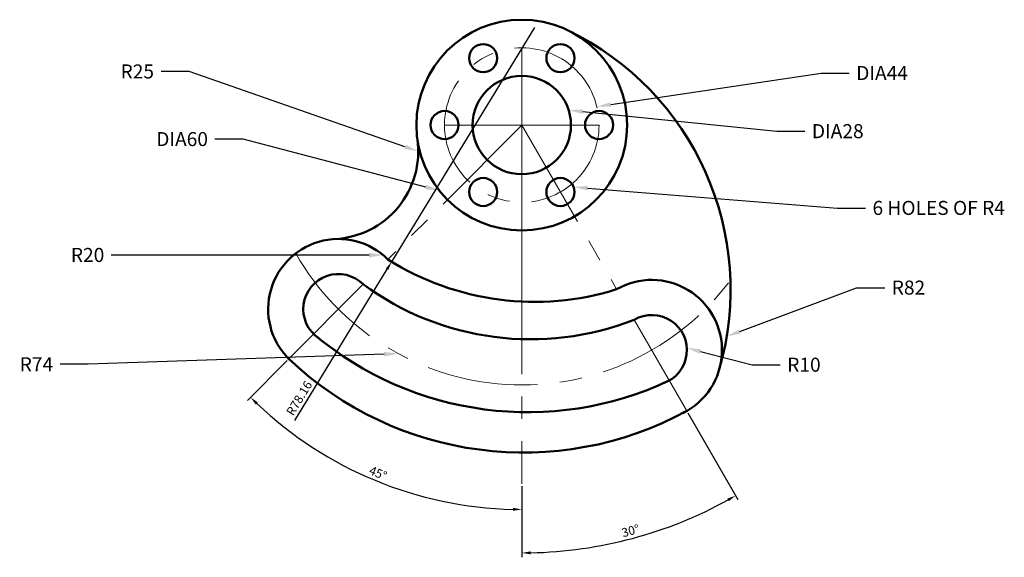
# Model space of a CAD drawing. Units: millimetres. Extents: x 3012 to 3292, y 2052 to 2205.
import ezdxf
from ezdxf import colors
from ezdxf.entities.mleader import LeaderData, LeaderLine
from ezdxf.math import Vec2, Vec3

# ---------------------------------------------------------------- set-up
doc = ezdxf.new("R2010")
doc.units = ezdxf.units.MM
doc.linetypes.add('CENTER', pattern=[50.8, 31.75, -6.35, 6.35, -6.35])
for name, color, linetype, lineweight in [('M-CNTR', 4, 'CENTER', 18), ('M-DIMS', 2, 'Continuous', 25), ('M-OUTL', 7, 'Continuous', 50)]:
    doc.layers.add(name, color=color, linetype=linetype, lineweight=lineweight)
doc.styles.get("Standard").update_dxf_attribs({"font": 'arial.ttf'})
doc.dimstyles.new('ISO-25', dxfattribs={"dimtxt": 2.5, "dimasz": 2.5, "dimexe": 1.25, "dimexo": 0.625, "dimtad": 1, "dimtxsty": 'Standard', "dimcen": 2.5, "dimadec": 0, "dimazin": 0, "dimtfac": 1, "dimtmove": 0, "dimatfit": 3, "dimfxl": 1, "dimarcsym": 0})

# ---------------------------------------------------------------- blocks, each defined once
blk = doc.blocks.new('*U1')
blk.add_circle((0, 0), 4)
blk = doc.blocks.new('*U2')
at = {"layer": 'M-OUTL', "color": 0, "linetype": 'ByBlock', "lineweight": -2, "transparency": 16777216}
for p, rotation in [((3143.61, 2193.94), 300), ((3165.61, 2193.94), 240), ((3176.61, 2174.89), 180), ((3143.61, 2155.83), 59.99999999999999), ((3165.61, 2155.83), 119.9999999999999)]:
    blk.add_blockref('*U1', p, dxfattribs=dict(at, rotation=rotation))
blk.add_blockref('*U1', (3132.61, 2174.89), dxfattribs=at)
blk = doc.blocks.new('*D3')
at = {"layer": 'Defpoints', "color": 0, "transparency": 16777216}
for p in [(3154.61, 2135.71), (3109.44, 2129.55), (3088.27, 2108.29), (3100.01, 2080.03), (3154.61, 2072.72)]:
    blk.add_point(p, dxfattribs=at)
at = {"layer": 'M-DIMS', "color": 0, "lineweight": -2, "transparency": 16777216}
for p, q in [((3087.83, 2107.85), (3076.49, 2096.46)), ((3154.61, 2072.1), (3154.61, 2064.19))]:
    blk.add_line(p, q, dxfattribs=at)
blk.add_arc((3154.61, 2174.89), 109.45, 226.4177, 268.6912, dxfattribs=at)
at = {"layer": 'M-DIMS', "color": 0, "transparency": 16777216}
for points in [[(3078.87, 2095.31), (3079.45, 2095.9), (3077.37, 2097.35)], [(3152.12, 2065.89), (3152.11, 2065.05), (3154.61, 2065.44)]]:
    blk.add_solid(points, dxfattribs=at)
at = {"layer": 'M-DIMS', "color": 0, "transparency": 16777216, "insert": (3113.55, 2075.49), "char_height": 2.5, "attachment_point": 5, "rotation": 337.5545}
blk.add_mtext('45°', dxfattribs=at)
blk = doc.blocks.new('*D4')
at = {"layer": 'Defpoints', "color": 0, "transparency": 16777216}
for p in [(3154.61, 2135.71), (3186.61, 2119.46), (3201.61, 2093.48), (3154.61, 2072.72), (3175.77, 2054.91)]:
    blk.add_point(p, dxfattribs=at)
at = {"layer": 'M-DIMS', "color": 0, "lineweight": -2, "transparency": 16777216}
for p, q in [((3201.93, 2092.94), (3216.15, 2068.3)), ((3154.61, 2072.1), (3154.61, 2051.81))]:
    blk.add_line(p, q, dxfattribs=at)
blk.add_arc((3154.61, 2174.89), 121.83, 271.1758, 298.8242, dxfattribs=at)
at = {"layer": 'M-DIMS', "color": 0, "transparency": 16777216}
for points in [[(3213.14, 2068.52), (3213.55, 2067.79), (3215.53, 2069.38)], [(3157.12, 2052.67), (3157.11, 2053.5), (3154.61, 2053.06)]]:
    blk.add_solid(points, dxfattribs=at)
at = {"layer": 'M-DIMS', "color": 0, "transparency": 16777216, "insert": (3185.65, 2059.05), "char_height": 2.5, "attachment_point": 5, "rotation": 15}
blk.add_mtext('30°', dxfattribs=at)
blk = doc.blocks.new('*D5')
at = {"layer": 'Defpoints', "color": 0, "transparency": 16777216}
for p in [(3158.25, 2202.71), (3117.55, 2135.98)]:
    blk.add_point(p, dxfattribs=at)
at = {"layer": 'M-DIMS', "color": 0, "lineweight": -2, "transparency": 16777216}
for p, q in [((3158.25, 2202.71), (3117.55, 2135.98)), ((3089.98, 2090.79), (3116.24, 2133.85))]:
    blk.add_line(p, q, dxfattribs=at)
at = {"layer": 'M-DIMS', "color": 0, "transparency": 16777216}
blk.add_solid([(3115.89, 2134.07), (3116.6, 2133.63), (3117.55, 2135.98)], dxfattribs=at)
at = {"layer": 'M-DIMS', "color": 0, "transparency": 16777216, "insert": (3091.5, 2096.94), "char_height": 2.5, "attachment_point": 5, "rotation": 58.6174}
blk.add_mtext('R78.16', dxfattribs=at)

msp = doc.modelspace()

# ---------------------------------------------------------------- linework, layer by layer
at = {"layer": 'M-CNTR'}
for p, q in [((3154.613, 2174.887), (3154.613, 2196.887)), ((3154.613, 2196.887), (3154.613, 2135.712)), ((3154.613, 2174.887), (3116.501, 2136.631)), ((3132.613, 2174.887), (3154.613, 2174.887)), ((3176.613, 2174.887), (3132.613, 2174.887)), ((3154.613, 2174.887), (3176.613, 2174.887)), ((3154.613, 2174.887), (3154.613, 2144.887)), ((3154.613, 2174.887), (3154.613, 2144.887)), ((3154.613, 2174.887), (3181.613, 2128.122)), ((3154.613, 2135.712), (3154.613, 2072.723)), ((3109.444, 2129.546), (3088.271, 2108.293)), ((3186.613, 2119.462), (3201.613, 2093.481))]:
    msp.add_line(p, q, dxfattribs=at)
msp.add_circle((3154.613, 2174.887), 22, dxfattribs=at)
msp.add_arc((3154.613, 2174.887), 74, 209.57604, 323.38645, dxfattribs=at)
at = {"layer": 'M-OUTL'}
for radius in [30, 14]:
    msp.add_circle((3154.613, 2174.887), radius, dxfattribs=at)
for centre, radius, start, end in [((3132.056, 2128.034), 82, 343.86196, 64.29192), ((3100.124, 2167.405), 25, 272.88172, 7.81873), ((3102.386, 2122.462), 20, 45.10891, 228.70551), ((3158.249, 2202.711), 78.163, 237.7166, 287.39231), ((3102.386, 2122.462), 10, 45.10887, 235.86184), ((3157.157, 2194.358), 80.481, 233.64021, 291.46869), ((3191.613, 2110.801), 20, 296.4034, 120), ((3191.613, 2110.801), 10, 289.24699, 119.99997), ((3156.305, 2187.837), 94.702, 229.91849, 295.19042), ((3155.129, 2178.838), 97.194, 226.53722, 298.57169)]:
    msp.add_arc(centre, radius, start, end, dxfattribs=at)

# ---------------------------------------------------------------- block references
msp.add_blockref('*U2', (0, 0), dxfattribs=at)

# ---------------------------------------------------------------- dimensions: what is measured, and where the dimension line sits
at = {"layer": 'M-DIMS'}
dim = msp.add_radius_dim(center=(3158.249, 2202.711), mpoint=(3117.546, 2135.983), dimstyle='ISO-25', override={"dimdec": 2, "dimlfac": 1, "dimrnd": 0, "dimzin": 0, "dimdsep": 46, "dimlunit": 2}, dxfattribs=at)
dim.commit()
dim.dimension.update_dxf_attribs({"geometry": '*D5', "text_midpoint": (3093.124, 2095.946), "dimtype": 164})
for base, line2, picture, middle in [((3100.01, 2080.035), ((3109.444, 2129.546), (3088.271, 2108.293)), '*D3', (3113.55, 2075.485)), ((3175.768, 2054.912), ((3186.613, 2119.462), (3201.613, 2093.481)), '*D4', (3185.651, 2059.049))]:
    dim = msp.add_angular_dim_2l(base=base, line1=((3154.613, 2135.712), (3154.613, 2072.723)), line2=line2, dimstyle='ISO-25', override={"dimclrd": 0, "dimclre": 0, "dimclrt": 0}, dxfattribs=at)
    dim.commit()
    dim.dimension.update_dxf_attribs({"geometry": picture, "text_midpoint": middle})

# ---------------------------------------------------------------- leaders
ml = msp.add_multileader_mtext('Standard', dxfattribs=at)
ml.set_content('R25', color=256)
ml.set_leader_properties()
ml.build(insert=Vec2(0, 0))
ctx = ml.context
ctx.base_point, ctx.plane_origin = Vec3(3038.297, 2190.12), Vec3(3125.124, 2167.405)
ctx.text_align_type = 2
notes = []
notes.append((ctx, [(0, (1, 1, 0), (3059.885, 2190.12), (-1, 0), 8, [(0, [(3125.124, 2167.405)], 0, [])])]))
ctx.mtext.insert, ctx.mtext.alignment, ctx.mtext.flow_direction = Vec3(3049.885, 2192.154), 3, 5
ml = msp.add_multileader_mtext('Standard', dxfattribs=at)
ml.set_content('DIA44', color=256)
ml.set_leader_properties()
ml.build(insert=Vec2(0, 0))
ctx = ml.context
ctx.base_point, ctx.plane_origin = Vec3(3247.839, 2189.704), Vec3(3175.977, 2180.137)
notes.append((ctx, [(0, (1, 1, 0), (3239.839, 2189.704), (1, 0), 8, [(0, [(3175.977, 2180.137)], 0, [])])]))
ctx.mtext.insert, ctx.mtext.flow_direction = Vec3(3249.839, 2191.704), 5
ml = msp.add_multileader_mtext('Standard', dxfattribs=at)
ml.set_content('DIA28', color=256)
ml.set_leader_properties()
ml.build(insert=Vec2(0, 0))
ctx = ml.context
ctx.base_point, ctx.plane_origin = Vec3(3235.215, 2173.117), Vec3(3167.956, 2179.123)
notes.append((ctx, [(0, (1, 1, 0), (3227.215, 2173.117), (1, 0), 8, [(0, [(3167.956, 2179.123)], 0, [])])]))
ctx.mtext.insert, ctx.mtext.flow_direction = Vec3(3237.215, 2175.151), 5
ml = msp.add_multileader_mtext('Standard', dxfattribs=at)
ml.set_content('DIA60', color=256)
ml.set_leader_properties()
ml.build(insert=Vec2(0, 0))
ctx = ml.context
ctx.base_point, ctx.plane_origin = Vec3(3048.415, 2170.855), Vec3(3131.123, 2156.226)
ctx.text_align_type = 2
notes.append((ctx, [(0, (1, 1, 0), (3075.248, 2170.855), (-1, 0), 8, [(0, [(3131.123, 2156.226)], 0, [])])]))
ctx.mtext.insert, ctx.mtext.alignment, ctx.mtext.flow_direction = Vec3(3065.248, 2172.889), 3, 5
ml = msp.add_multileader_mtext('Standard', dxfattribs=at)
ml.set_content('6 HOLES OF R4', color=256)
ml.set_leader_properties()
ml.build(insert=Vec2(0, 0))
ctx = ml.context
ctx.base_point, ctx.plane_origin = Vec3(3252.472, 2151.263), Vec3(3169.356, 2157.245)
notes.append((ctx, [(0, (1, 1, 0), (3244.472, 2151.263), (1, 0), 8, [(0, [(3169.356, 2157.245)], 0, [])])]))
ctx.mtext.insert, ctx.mtext.flow_direction = Vec3(3254.472, 2153.297), 5
ml = msp.add_multileader_mtext('Standard', dxfattribs=at)
ml.set_content('R20', color=256)
ml.set_leader_properties()
ml.build(insert=Vec2(0, 0))
ctx = ml.context
ctx.base_point, ctx.plane_origin = Vec3(3024.185, 2137.863), Vec3(3115.146, 2137.863)
ctx.text_align_type = 2
notes.append((ctx, [(0, (1, 1, 0), (3045.729, 2137.863), (-1, 0), 8, [(0, [(3115.146, 2137.863)], 0, [])])]))
ctx.mtext.insert, ctx.mtext.alignment, ctx.mtext.flow_direction = Vec3(3035.729, 2139.897), 3, 5
ml = msp.add_multileader_mtext('Standard', dxfattribs=at)
ml.set_content('R82', color=256)
ml.set_leader_properties()
ml.build(insert=Vec2(0, 0))
ctx = ml.context
ctx.base_point, ctx.plane_origin = Vec3(3257.951, 2128.571), Vec3(3212.964, 2114.7)
notes.append((ctx, [(0, (1, 1, 0), (3249.951, 2128.571), (1, 0), 8, [(0, [(3212.964, 2114.7)], 0, [])])]))
ctx.mtext.insert, ctx.mtext.flow_direction = Vec3(3259.951, 2130.605), 5
ml = msp.add_multileader_mtext('Standard', dxfattribs=at)
ml.set_content('R10', color=256)
ml.set_leader_properties()
ml.build(insert=Vec2(0, 0))
ctx = ml.context
ctx.base_point, ctx.plane_origin = Vec3(3228.189, 2106.618), Vec3(3201.593, 2111.425)
notes.append((ctx, [(0, (1, 1, 0), (3220.189, 2106.618), (1, 0), 8, [(0, [(3201.593, 2111.425)], 0, [])])]))
ctx.mtext.insert, ctx.mtext.flow_direction = Vec3(3230.189, 2108.652), 5
ml = msp.add_multileader_mtext('Standard', dxfattribs=at)
ml.set_content('R74', color=256)
ml.set_leader_properties()
ml.build(insert=Vec2(0, 0))
ctx = ml.context
ctx.base_point, ctx.plane_origin = Vec3(3009.615, 2106.767), Vec3(3119.431, 2109.785)
ctx.text_align_type = 2
notes.append((ctx, [(0, (1, 1, 0), (3031.157, 2106.767), (-1, 0), 8, [(0, [(3119.431, 2109.785)], 0, [])])]))
ctx.mtext.insert, ctx.mtext.alignment, ctx.mtext.flow_direction = Vec3(3021.157, 2108.767), 3, 5
for ctx, leaders in notes:
    for number, flags, end, landing, length, lines in leaders:
        leader = LeaderData()
        leader.index, (leader.has_last_leader_line, leader.has_dogleg_vector, leader.attachment_direction) = number, flags
        leader.last_leader_point, leader.dogleg_vector, leader.dogleg_length = Vec3(end), Vec3(landing), length
        for number, points, colour, breaks in lines:
            line = LeaderLine()
            line.index, line.vertices, line.color, line.breaks = number, Vec3.list(points), colors.encode_raw_color(colour), breaks
            leader.lines.append(line)
        ctx.leaders.append(leader)

doc.saveas('drawing.dxf')
